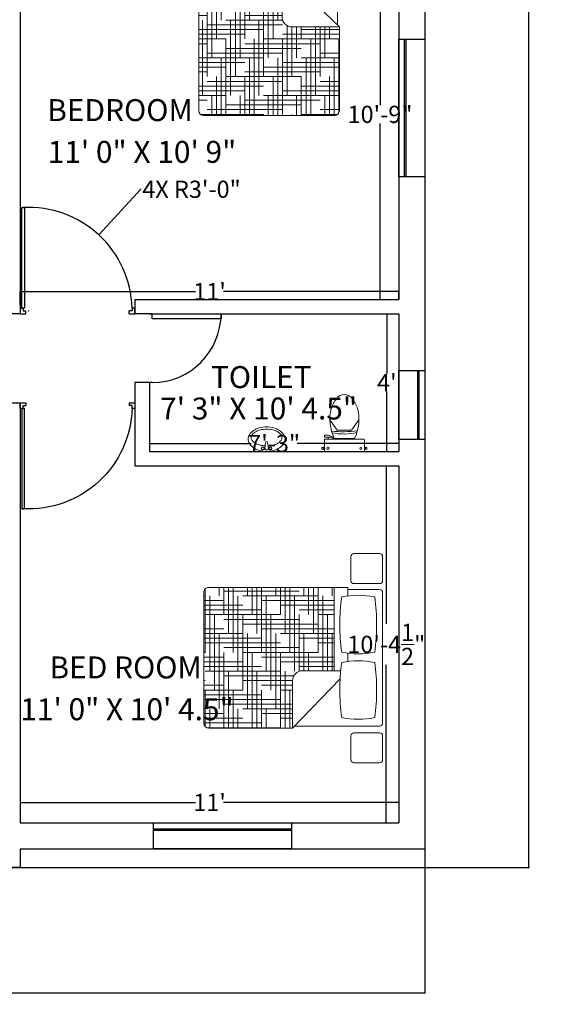
# Model space of a CAD drawing. Units: inches. Extents: x -113 to 5399, y -1393 to 3302.
# Tile 26 of 40: x 3982 to 4170, y -154 to 189. Entities that reach past the tile are written whole.
import ezdxf

# ---------------------------------------------------------------- set-up
doc = ezdxf.new("R2010")
doc.units = ezdxf.units.IN
doc.header["$MEASUREMENT"] = 0
for name, color, linetype, lineweight in [('A-ANNO-DIMS', 254, 'Continuous', 18), ('A-AREA-IDEN', 4, 'Continuous', 18), ('A-FLOR-FIXT', 8, 'Continuous', 18), ('doors', 2, 'Continuous', 25), ('furniture', 131, 'Continuous', 18), ('walls', 1, 'Continuous', 25), ('windows', 3, 'Continuous', 25)]:
    doc.layers.add(name, color=color, linetype=linetype, lineweight=lineweight)
doc.layers.add('A-GLAZ-PATT', color=85, linetype='Continuous', lineweight=13, true_color=0x58ba48)
doc.styles.get("Standard").update_dxf_attribs({"font": 'arial.ttf'})
doc.dimstyles.get("Standard").update_dxf_attribs({"dimtxt": 6, "dimasz": 0.18, "dimexe": 0.18, "dimexo": 0.0625, "dimgap": 0.09, "dimtad": 0, "dimtih": 1, "dimtoh": 1, "dimdec": 1, "dimzin": 0, "dimdsep": 46, "dimlunit": 4, "dimtxsty": 'Standard', "dimblk": 'ARCHTICK', "dimcen": 0.09, "dimadec": 0, "dimazin": 0, "dimtfac": 1, "dimtdec": 1, "dimtofl": 0, "dimtmove": 0, "dimatfit": 3, "dimfxl": 1, "dimtolj": 1, "dimtzin": 0, "dimarcsym": 0})

# ---------------------------------------------------------------- blocks, each defined once
blk = doc.blocks.new('*U2')
for p, q in [((0, 0), (0, -6)), ((24, 0), (24, -6))]:
    blk.add_line(p, q)
blk.add_lwpolyline([(0, 0), (0, 24), (1.75, 24), (1.75, 0)], close=True)
blk.add_arc((0, 0), 24, 0, 90)
blk = doc.blocks.new('*X4')
at = {"color": 0}
for p, q in [((4.3594, 18.5625), (4.3594, 18.6457)), ((4.5, 18), (4.5, 18.6457)), ((4.5469, 18.1875), (4.5469, 18.6457)), ((4.5938, 18.375), (4.5938, 18.6457)), ((4.6406, 18.5625), (4.6406, 18.6457)), ((4.7812, 18), (4.7812, 18.6457)), ((4.8281, 18.1875), (4.8281, 18.6457)), ((4.875, 18.375), (4.875, 18.6457)), ((4.9219, 18.5625), (4.9219, 18.6457)), ((5.0625, 18), (5.0625, 18.6457)), ((5.1094, 18.1875), (5.1094, 18.6457)), ((5.1562, 18.375), (5.1562, 18.6457)), ((5.2031, 18.5625), (5.2031, 18.6457)), ((5.3438, 18), (5.3438, 18.6457)), ((5.3906, 18.1875), (5.3906, 18.6457)), ((5.4375, 18.375), (5.4375, 18.6457)), ((5.4844, 18.5625), (5.4844, 18.6457)), ((5.625, 18), (5.625, 18.6287)), ((4.4531, 17.8169), (4.4531, 18.5625)), ((4.5, 18.5625), (5.25, 18.5625)), ((4.6875, 18.6094), (5.4375, 18.6094)), ((4.7344, 17.8125), (4.7344, 18.5625)), ((5.0156, 17.8125), (5.0156, 18.5625)), ((5.2969, 17.8125), (5.2969, 18.5625)), ((5.5781, 17.8125), (5.5781, 18.5625)), ((5.625, 18.5625), (5.6375, 18.5625)), ((4.3395, 18.5156), (5.0625, 18.5156)), ((4.3395, 18.4688), (4.875, 18.4688)), ((5.25, 18.4688), (5.6375, 18.4688)), ((5.4375, 18.5156), (5.6375, 18.5156)), ((4.3395, 18.4219), (4.6875, 18.4219)), ((4.3395, 18.375), (4.5, 18.375)), ((4.4062, 17.8169), (4.4062, 18.375)), ((4.6875, 17.8114), (4.6875, 18.375)), ((4.6875, 18.3281), (5.4375, 18.3281)), ((4.875, 18.375), (5.625, 18.375)), ((4.9688, 17.625), (4.9688, 18.375)), ((5.0625, 18.4219), (5.6375, 18.4219)), ((5.25, 17.625), (5.25, 18.375)), ((5.5312, 17.625), (5.5312, 18.375)), ((4.3395, 18.2344), (5.0625, 18.2344)), ((4.5, 18.2812), (5.25, 18.2812)), ((5.4375, 18.2344), (5.6375, 18.2344)), ((5.625, 18.2812), (5.6375, 18.2812)), ((4.3395, 18.1875), (4.875, 18.1875)), ((4.3395, 18.1406), (4.6875, 18.1406)), ((4.3594, 17.8169), (4.3594, 18.1875)), ((4.6406, 17.8169), (4.6406, 18.1875)), ((4.9219, 17.4375), (4.9219, 18.1875)), ((5.0625, 18.1406), (5.6375, 18.1406)), ((5.2031, 17.4375), (5.2031, 18.1875)), ((5.25, 18.1875), (5.6375, 18.1875)), ((5.4844, 17.4375), (5.4844, 18.1875)), ((4.3395, 18.0938), (4.5, 18.0938)), ((4.6875, 18.0469), (5.4375, 18.0469)), ((4.875, 18.0938), (5.625, 18.0938)), ((4.3395, 17.9531), (5.0625, 17.9531)), ((4.5, 18), (5.25, 18)), ((4.5938, 17.8169), (4.5938, 18)), ((4.875, 17.25), (4.875, 18)), ((5.1562, 17.25), (5.1562, 18)), ((5.4375, 17.25), (5.4375, 18)), ((5.4375, 17.9531), (5.6375, 17.9531)), ((5.625, 18), (5.6375, 18)), ((4.3395, 17.9062), (4.875, 17.9062)), ((4.3395, 17.8594), (4.6875, 17.8594)), ((5.0625, 17.8594), (5.6375, 17.8594)), ((5.25, 17.9062), (5.6375, 17.9062)), ((4.7421, 17.7656), (5.4375, 17.7656)), ((4.8281, 17.2457), (4.8281, 17.8125)), ((4.875, 17.8125), (5.625, 17.8125)), ((5.1094, 17.2457), (5.1094, 17.8125)), ((5.3906, 17.2457), (5.3906, 17.8125)), ((4.7548, 17.7188), (5.25, 17.7188)), ((4.7548, 17.6719), (5.0625, 17.6719)), ((5.4375, 17.6719), (5.6375, 17.6719)), ((5.625, 17.7188), (5.6375, 17.7188)), ((4.7548, 17.625), (4.875, 17.625)), ((4.7812, 17.2457), (4.7812, 17.625)), ((5.0625, 17.2457), (5.0625, 17.625)), ((5.0625, 17.5781), (5.6375, 17.5781)), ((5.25, 17.625), (5.6375, 17.625)), ((5.3438, 17.2457), (5.3438, 17.625)), ((5.625, 17.2627), (5.625, 17.625)), ((4.7548, 17.4844), (5.4375, 17.4844)), ((4.875, 17.5312), (5.625, 17.5312)), ((4.7548, 17.4375), (5.25, 17.4375)), ((4.7548, 17.3906), (5.0625, 17.3906)), ((5.0156, 17.2457), (5.0156, 17.4375)), ((5.2969, 17.2457), (5.2969, 17.4375)), ((5.4375, 17.3906), (5.6375, 17.3906)), ((5.5781, 17.2457), (5.5781, 17.4375)), ((5.625, 17.4375), (5.6375, 17.4375)), ((4.7548, 17.3438), (4.875, 17.3438)), ((4.875, 17.25), (5.6077, 17.25)), ((4.9688, 17.2457), (4.9688, 17.25)), ((5.0625, 17.2969), (5.6375, 17.2969)), ((5.25, 17.3438), (5.6375, 17.3438)), ((5.25, 17.2457), (5.25, 17.25)), ((5.5312, 17.2457), (5.5312, 17.25))]:
    blk.add_line(p, q, dxfattribs=at)
blk = doc.blocks.new('MAT-P01')
for p, q in [((-0.0213, 0.8164), (-0.0213, 0.5605)), ((0.0087, 0.8464), (0.2471, 0.8464)), ((0.2771, 0.8164), (0.2771, 0.5605)), ((0.3437, 0.8164), (0.3437, -0.0316)), ((0.3737, 0.8464), (1.6737, 0.8464)), ((1.7037, 0.8164), (1.7037, 0.5005)), ((1.7622, 0.8164), (1.7622, 0.5605)), ((1.7922, 0.8464), (2.0306, 0.8464)), ((2.0606, 0.8164), (2.0606, 0.5605)), ((0.0087, 0.5305), (0.2471, 0.5305)), ((0.9879, 0.5005), (1.0693, 0.5005)), ((1.6393, 0.5005), (1.7237, 0.5005)), ((1.7237, 0.5005), (1.7237, -0.8836)), ((1.7922, 0.5305), (2.0306, 0.5305)), ((0.8146, 0.423), (0.3237, -0.0509)), ((0.8949, 0.4293), (0.8949, 0.0491)), ((0.8949, 0.3643), (1.7237, 0.3643)), ((0.8949, 0.3643), (0.8949, 0.0491)), ((0.8949, 0.3643), (1.7237, 0.3643)), ((1.7237, 0.3643), (1.7237, -0.8836)), ((0.3237, -0.0509), (0.7949, -0.0509)), ((0.3237, -0.0509), (0.3237, -0.8836)), ((0.3737, -0.9336), (1.6737, -0.9336))]:
    blk.add_line(p, q)
for centre, radius, start, end in [((0.0087, 0.8164), 0.03, 90, 180), ((0.2471, 0.8164), 0.03, 0, 90), ((0.3737, 0.8164), 0.03, 90, 180), ((0.7029, -1.1436), 1.9306, 81.81622, 98.18378), ((1.3543, -1.1436), 1.9306, 81.81622, 98.18378), ((1.6737, 0.8164), 0.03, 0, 90), ((1.7922, 0.8164), 0.03, 90, 180), ((2.0306, 0.8164), 0.03, 0, 90), ((1.2251, 0.6034), 0.8138, 168.37298, 191.62702), ((0.1806, 0.6034), 0.8138, 348.37298, 11.62702), ((1.8766, 0.6034), 0.8138, 168.37298, 191.62702), ((0.8321, 0.6034), 0.8138, 348.37298, 11.62702), ((0.0087, 0.5605), 0.03, 180, 270), ((0.2471, 0.5605), 0.03, 270, 0), ((1.7922, 0.5605), 0.03, 180, 270), ((2.0306, 0.5605), 0.03, 270, 0), ((0.7029, 2.3504), 1.9306, 261.81622, 278.18378), ((1.3543, 2.3504), 1.9306, 261.81622, 278.18378), ((0.7949, 0.0491), 0.1, 270, 0), ((0.3737, -0.8836), 0.05, 180, 270), ((1.6737, -0.8836), 0.05, 270, 0)]:
    blk.add_arc(centre, radius, start, end)
at = {"rotation": 270}
blk.add_blockref('*X4', (-16.9221, 4.7038), dxfattribs=at)
blk = doc.blocks.new('toilet-3')
at = {"color": 0, "linetype": 'ByBlock'}
for p, q in [((-0.281, -0.05), (-0.281, -0.069)), ((-0.281, -0.05), (-0.261, -0.05)), ((-0.281, -0.069), (-0.261, -0.069)), ((-0.261, -0.047), (-0.261, -0.072)), ((-0.261, -0.047), (-0.251, -0.047)), ((-0.261, -0.072), (-0.251, -0.072)), ((-0.251, -0.047), (-0.251, -0.072)), ((-0.25, -0.03), (-0.25, -0.165)), ((0.24, -0.02), (-0.24, -0.02)), ((0.25, -0.03), (0.25, -0.165)), ((0.261, -0.047), (0.251, -0.047)), ((0.251, -0.047), (0.251, -0.072)), ((0.261, -0.072), (0.251, -0.072)), ((0.261, -0.047), (0.261, -0.072)), ((0.281, -0.05), (0.261, -0.05)), ((0.281, -0.069), (0.261, -0.069)), ((0.281, -0.05), (0.281, -0.069)), ((-0.144, -0.2), (-0.25, -0.2)), ((-0.25, -0.2), (-0.25, -0.222)), ((-0.198, -0.222), (-0.25, -0.222)), ((0.24, -0.175), (-0.24, -0.175)), ((-0.202, -0.2), (-0.202, -0.175)), ((-0.198, -0.222), (-0.16, -0.207)), ((-0.16, -0.207), (-0.16, -0.2)), ((-0.144, -0.2), (-0.144, -0.175)), ((0.125, -0.182), (-0.125, -0.182)), ((-0.089, -0.287), (-0.18, -0.415)), ((0.089, -0.287), (-0.089, -0.287)), ((0.089, -0.287), (0.18, -0.415))]:
    blk.add_line(p, q, dxfattribs=at)
for centre in [(-0.205, -0.059), (0.205, -0.059)]:
    blk.add_circle(centre, 0.0125, dxfattribs=at)
for centre, radius, start, end in [((-0.24, -0.03), 0.01, 90, 180), ((0.24, -0.03), 0.01, 0, 90), ((-0.24, -0.165), 0.01, 180, 270), ((0.376, -0.424), 0.557, 154.2321, 193.6755), ((-0.005, -0.896), 0.659, 75.9276, 103.0204), ((-0.376, -0.424), 0.557, 346.3245, 25.7679), ((0.24, -0.165), 0.01, 270, 0), ((-0.013, -1.787), 1.521, 83.4552, 95.5271), ((0.262, -0.406), 0.452, 199.2942, 217.2549), ((-0.265, -0.4), 0.457, 322.2382, 340.1051), ((-0.001, -0.609), 0.12, 216.3794, 323.6206)]:
    blk.add_arc(centre, radius, start, end, dxfattribs=at)
blk = doc.blocks.new('wash-6')
at = {"color": 0, "linetype": 'ByBlock'}
for p, q in [((-0.036, -0.063), (-0.021, -0.18)), ((0.036, -0.063), (0.021, -0.18))]:
    blk.add_line(p, q, dxfattribs=at)
for centre, radius in [((-0.075, -0.062), 0.0325), ((-0.075, -0.062), 0.0263), ((0.075, -0.062), 0.0325), ((0.075, -0.062), 0.0263)]:
    blk.add_circle(centre, radius, dxfattribs=at)
for centre, radius, start, end in [((0, -0.56), 0.56, 90, 105.4371), ((-0.204, -0.25), 0.17, 148.1465, 180), ((-0.107, -0.311), 0.285, 123.6901, 148.1465), ((-0.114, -0.361), 0.225, 118.369, 142.5096), ((-0.042, -0.407), 0.401, 105.4371, 123.6901), ((-0.045, -0.488), 0.37, 102.6081, 118.369), ((0, -0.69), 0.576, 92.9466, 102.6081), ((0, -0.063), 0.0361, 0, 180), ((0, -0.18), 0.0215, 180, 0), ((0, -0.56), 0.56, 74.5629, 90), ((0, -0.69), 0.576, 77.3919, 87.0534), ((0.045, -0.488), 0.37, 61.631, 77.3919), ((0.042, -0.407), 0.401, 56.3099, 74.5629), ((0.114, -0.361), 0.225, 37.4904, 61.631), ((0.107, -0.311), 0.285, 31.8535, 56.3099), ((0.204, -0.25), 0.17, 0, 31.8535), ((-0.204, -0.25), 0.17, 180, 211.8535), ((-0.107, -0.189), 0.285, 211.8535, 236.3099), ((-0.217, -0.282), 0.0954, 142.5096, 180), ((-0.217, -0.282), 0.0954, 180, 217.4904), ((-0.114, -0.203), 0.225, 217.4904, 241.631), ((0.114, -0.203), 0.225, 298.369, 322.5096), ((0.107, -0.189), 0.285, 303.6901, 328.1465), ((0.217, -0.282), 0.0954, 0, 37.4904), ((0.217, -0.282), 0.0954, 322.5096, 0), ((0.204, -0.25), 0.17, 328.1465, 0), ((-0.042, -0.092), 0.401, 236.3099, 254.5629), ((-0.045, -0.076), 0.37, 241.631, 257.3919), ((0, 0.06), 0.56, 254.5629, 270), ((0, 0.125), 0.576, 257.3919, 270), ((0, 0.125), 0.576, 270, 282.6081), ((0, 0.06), 0.56, 270, 285.4371), ((0.045, -0.076), 0.37, 282.6081, 298.369), ((0.042, -0.092), 0.401, 285.4371, 303.6901)]:
    blk.add_arc(centre, radius, start, end, dxfattribs=at)
blk = doc.blocks.new('_ArchTick')
at = {"color": 0, "linetype": 'ByBlock', "const_width": 0.15}
blk.add_lwpolyline([(-0.5, -0.5), (0.5, 0.5)], dxfattribs=at)
blk = doc.blocks.new('*D99')
at = {"layer": 'A-ANNO-DIMS', "color": 0, "lineweight": -2, "transparency": 16777216}
for p, q in [((3689.73, -100.29), (3689.73, -150.66)), ((4122.73, -100.29), (4122.73, -150.66)), ((3689.73, -150.48), (3895.84, -150.48)), ((4122.73, -150.48), (3916.62, -150.48))]:
    blk.add_line(p, q, dxfattribs=at)
at = {"layer": 'Defpoints', "color": 0, "transparency": 16777216}
for p in [(3689.73, -100.22), (4122.73, -100.22), (4122.73, -150.48)]:
    blk.add_point(p, dxfattribs=at)
at = {"layer": 'A-ANNO-DIMS', "color": 0, "lineweight": -2, "transparency": 16777216, "xscale": 0.18, "yscale": 0.18, "zscale": 0.18, "rotation": 180}
blk.add_blockref('_ArchTick', (3689.73, -150.48), dxfattribs=at)
at = {"layer": 'A-ANNO-DIMS', "color": 0, "lineweight": -2, "transparency": 16777216, "xscale": 0.18, "yscale": 0.18, "zscale": 0.18}
blk.add_blockref('_ArchTick', (4122.73, -150.48), dxfattribs=at)
at = {"layer": 'A-ANNO-DIMS', "color": 0, "transparency": 16777216, "insert": (3906.23, -150.48), "char_height": 6, "attachment_point": 5}
blk.add_mtext('\\A1;36\'-1"', dxfattribs=at)
blk = doc.blocks.new('*D103')
at = {"layer": 'A-ANNO-DIMS', "color": 0, "lineweight": -2, "transparency": 16777216}
for p, q in [((4107.42, 220.28), (4106.96, 220.28)), ((4107.14, 220.28), (4107.14, 158.93)), ((4107.14, 91.28), (4107.14, 152.62)), ((4107.42, 91.28), (4106.96, 91.28))]:
    blk.add_line(p, q, dxfattribs=at)
at = {"layer": 'Defpoints', "color": 0, "transparency": 16777216}
for p in [(4107.48, 220.28), (4107.14, 91.28), (4107.48, 91.28)]:
    blk.add_point(p, dxfattribs=at)
at = {"layer": 'A-ANNO-DIMS', "color": 0, "lineweight": -2, "transparency": 16777216, "xscale": 0.18, "yscale": 0.18, "zscale": 0.18}
for p, rotation in [((4107.14, 220.28), 90), ((4107.14, 91.28), 270)]:
    blk.add_blockref('_ArchTick', p, dxfattribs=dict(at, rotation=rotation))
at = {"layer": 'A-ANNO-DIMS', "color": 0, "transparency": 16777216, "insert": (4107.14, 155.78), "char_height": 6, "attachment_point": 5}
blk.add_mtext('\\A1;10\'-9"', dxfattribs=at)
blk = doc.blocks.new('*D104')
at = {"layer": 'A-ANNO-DIMS', "color": 0, "lineweight": -2, "transparency": 16777216}
for p, q in [((3981.73, 89.33), (3981.73, 94.18)), ((3981.73, 94), (4042.83, 94)), ((4113.73, 94), (4052.63, 94)), ((4113.73, 91.34), (4113.73, 94.18))]:
    blk.add_line(p, q, dxfattribs=at)
at = {"layer": 'Defpoints', "color": 0, "transparency": 16777216}
for p in [(4113.73, 94), (3981.73, 89.26), (4113.73, 91.28)]:
    blk.add_point(p, dxfattribs=at)
at = {"layer": 'A-ANNO-DIMS', "color": 0, "lineweight": -2, "transparency": 16777216, "xscale": 0.18, "yscale": 0.18, "zscale": 0.18, "rotation": 180}
blk.add_blockref('_ArchTick', (3981.73, 94), dxfattribs=at)
at = {"layer": 'A-ANNO-DIMS', "color": 0, "lineweight": -2, "transparency": 16777216, "xscale": 0.18, "yscale": 0.18, "zscale": 0.18}
blk.add_blockref('_ArchTick', (4113.73, 94), dxfattribs=at)
at = {"layer": 'A-ANNO-DIMS', "color": 0, "transparency": 16777216, "insert": (4047.73, 94), "char_height": 6, "attachment_point": 5}
blk.add_mtext("\\A1;11'", dxfattribs=at)
blk = doc.blocks.new('*D105')
at = {"layer": 'A-ANNO-DIMS', "color": 0, "lineweight": -2, "transparency": 16777216}
for p, q in [((4109.32, 86.28), (4109.69, 86.28)), ((4109.51, 86.28), (4109.51, 65.37)), ((4109.51, 38.28), (4109.51, 59.19)), ((4109.32, 38.28), (4109.69, 38.28))]:
    blk.add_line(p, q, dxfattribs=at)
at = {"layer": 'Defpoints', "color": 0, "transparency": 16777216}
for p in [(4109.25, 86.28), (4109.25, 38.28), (4109.51, 38.28)]:
    blk.add_point(p, dxfattribs=at)
at = {"layer": 'A-ANNO-DIMS', "color": 0, "lineweight": -2, "transparency": 16777216, "xscale": 0.18, "yscale": 0.18, "zscale": 0.18}
for p, rotation in [((4109.51, 86.28), 90), ((4109.51, 38.28), 270)]:
    blk.add_blockref('_ArchTick', p, dxfattribs=dict(at, rotation=rotation))
at = {"layer": 'A-ANNO-DIMS', "color": 0, "transparency": 16777216, "insert": (4109.51, 62.28), "char_height": 6, "attachment_point": 5}
blk.add_mtext("\\A1;4'", dxfattribs=at)
blk = doc.blocks.new('*D106')
at = {"layer": 'A-ANNO-DIMS', "color": 0, "lineweight": -2, "transparency": 16777216}
for p, q in [((4026.73, 41.09), (4026.73, 41.21)), ((4113.73, 41.09), (4113.73, 41.21)), ((4026.73, 41.03), (4062.19, 41.03)), ((4113.73, 41.03), (4078.27, 41.03))]:
    blk.add_line(p, q, dxfattribs=at)
at = {"layer": 'Defpoints', "color": 0, "transparency": 16777216}
for p in [(4026.73, 41.03), (4113.73, 41.03), (4113.73, 41.03)]:
    blk.add_point(p, dxfattribs=at)
at = {"layer": 'A-ANNO-DIMS', "color": 0, "lineweight": -2, "transparency": 16777216, "xscale": 0.18, "yscale": 0.18, "zscale": 0.18, "rotation": 180}
blk.add_blockref('_ArchTick', (4026.73, 41.03), dxfattribs=at)
at = {"layer": 'A-ANNO-DIMS', "color": 0, "lineweight": -2, "transparency": 16777216, "xscale": 0.18, "yscale": 0.18, "zscale": 0.18}
blk.add_blockref('_ArchTick', (4113.73, 41.03), dxfattribs=at)
at = {"layer": 'A-ANNO-DIMS', "color": 0, "transparency": 16777216, "insert": (4070.23, 41.03), "char_height": 6, "attachment_point": 5}
blk.add_mtext('\\A1;7\'-3"', dxfattribs=at)
blk = doc.blocks.new('*D119')
at = {"layer": 'A-ANNO-DIMS', "color": 0, "lineweight": -2, "transparency": 16777216}
for p, q in [((4108.21, 33.28), (4109.51, 33.28)), ((4109.33, 33.28), (4109.33, -21.81)), ((4109.33, -91.22), (4109.33, -36.14)), ((4108.21, -91.22), (4109.51, -91.22))]:
    blk.add_line(p, q, dxfattribs=at)
at = {"layer": 'Defpoints', "color": 0, "transparency": 16777216}
for p in [(4108.15, 33.28), (4108.15, -91.22), (4109.33, -91.22)]:
    blk.add_point(p, dxfattribs=at)
at = {"layer": 'A-ANNO-DIMS', "color": 0, "lineweight": -2, "transparency": 16777216, "xscale": 0.18, "yscale": 0.18, "zscale": 0.18}
for p, rotation in [((4109.33, 33.28), 90), ((4109.33, -91.22), 270)]:
    blk.add_blockref('_ArchTick', p, dxfattribs=dict(at, rotation=rotation))
at = {"layer": 'A-ANNO-DIMS', "color": 0, "transparency": 16777216, "insert": (4109.33, -28.97), "char_height": 6, "attachment_point": 5}
blk.add_mtext('\\A1;10\'-4{\\H1x;\\S1/2;}"', dxfattribs=at)
blk = doc.blocks.new('*D120')
at = {"layer": 'A-ANNO-DIMS', "color": 0, "lineweight": -2, "transparency": 16777216}
for p, q in [((3981.73, -83.95), (3981.73, -84.23)), ((3981.73, -84.05), (4042.83, -84.05)), ((4113.73, -84.05), (4052.63, -84.05)), ((4113.73, -83.95), (4113.73, -84.23))]:
    blk.add_line(p, q, dxfattribs=at)
at = {"layer": 'Defpoints', "color": 0, "transparency": 16777216}
for p in [(3981.73, -83.88), (4113.73, -83.88), (4113.73, -84.05)]:
    blk.add_point(p, dxfattribs=at)
at = {"layer": 'A-ANNO-DIMS', "color": 0, "lineweight": -2, "transparency": 16777216, "xscale": 0.18, "yscale": 0.18, "zscale": 0.18, "rotation": 180}
blk.add_blockref('_ArchTick', (3981.73, -84.05), dxfattribs=at)
at = {"layer": 'A-ANNO-DIMS', "color": 0, "lineweight": -2, "transparency": 16777216, "xscale": 0.18, "yscale": 0.18, "zscale": 0.18}
blk.add_blockref('_ArchTick', (4113.73, -84.05), dxfattribs=at)
at = {"layer": 'A-ANNO-DIMS', "color": 0, "transparency": 16777216, "insert": (4047.73, -84.05), "char_height": 6, "attachment_point": 5}
blk.add_mtext("\\A1;11'", dxfattribs=at)
blk = doc.blocks.new('WIN-PLAN-48IN')
h = blk.add_hatch(color=256)
h.dxf.hatch_style = 1
h.paths.add_polyline_path([(48, 2.5), (0, 2.5), (0, 2), (48, 2)])
for p, q in [((0, 9), (48, 9)), ((0, 0), (0, 9)), ((48, 9), (48, 0)), ((48, 2.5), (0, 2.5)), ((48, 2), (0, 2)), ((48, 0), (0, 0))]:
    blk.add_line(p, q)
blk = doc.blocks.new('DOOR-SINGLE-36IN-PLAN')
for p, q in [((0.5, 2), (0.5, 36.98)), ((0.5, 36.98), (1.5, 36.98)), ((1.5, 36.98), (1.5, 2)), ((0, 2), (0, 0)), ((0, 2), (1.04, 2)), ((1.5, 2), (0.5, 2)), ((1.04, 2), (1.04, 0.98)), ((1.04, 0.98), (2, 0.98)), ((2, 0), (2, 0.98)), ((38.96, 0.98), (38, 0.98)), ((38, 0), (38, 0.98)), ((40, 2), (38.96, 2)), ((38.96, 2), (38.96, 0.98)), ((40, 0), (40, 2)), ((0, 0), (2, 0)), ((0, 0), (2, 0)), ((38, 0), (40, 0))]:
    blk.add_line(p, q)
blk.add_arc((2.94, 0.99), 36.04, 1.6003, 93.0893)
blk = doc.blocks.new('*D210')
at = {"layer": 'A-ANNO-DIMS', "color": 0, "lineweight": -2, "transparency": 16777216}
for p, q in [((3839.79, 561.28), (4159.21, 561.28)), ((4159.03, 561.28), (4159.03, 230.43)), ((4159.03, -106.72), (4159.03, 224.12)), ((3839.79, -106.72), (4159.21, -106.72))]:
    blk.add_line(p, q, dxfattribs=at)
at = {"layer": 'Defpoints', "color": 0, "transparency": 16777216}
for p in [(3839.73, 561.28), (4159.03, 561.28), (3839.73, -106.72)]:
    blk.add_point(p, dxfattribs=at)
at = {"layer": 'A-ANNO-DIMS', "color": 0, "lineweight": -2, "transparency": 16777216, "xscale": 0.18, "yscale": 0.18, "zscale": 0.18}
for p, rotation in [((4159.03, 561.28), 90), ((4159.03, -106.72), 270)]:
    blk.add_blockref('_ArchTick', p, dxfattribs=dict(at, rotation=rotation))
at = {"layer": 'A-ANNO-DIMS', "color": 0, "transparency": 16777216, "insert": (4159.03, 227.28), "char_height": 6, "attachment_point": 5}
blk.add_mtext('\\A1;55\'-8"', dxfattribs=at)
blk = doc.blocks.new('*D240')
at = {"layer": 'A-ANNO-DIMS', "color": 0, "lineweight": -2, "transparency": 16777216}
for p, q in [((4023.74, 129.67), (4009.09, 113.77)), ((4023.92, 129.67), (4023.74, 129.67)), ((3984.58, 87.27), (3984.76, 87.27)), ((3984.67, 87.18), (3984.67, 87.36))]:
    blk.add_line(p, q, dxfattribs=at)
at = {"layer": 'Defpoints', "color": 0, "transparency": 16777216}
for p in [(4009.09, 113.77), (3984.67, 87.27)]:
    blk.add_point(p, dxfattribs=at)
at = {"layer": 'A-ANNO-DIMS', "color": 0, "lineweight": -2, "transparency": 16777216, "xscale": 0.18, "yscale": 0.18, "zscale": 0.18, "rotation": 227.3452027332481}
blk.add_blockref('_ArchTick', (4009.09, 113.77), dxfattribs=at)
at = {"layer": 'A-ANNO-DIMS', "color": 0, "transparency": 16777216, "insert": (4041.42, 129.67), "char_height": 6, "attachment_point": 5}
blk.add_mtext('\\A1;4X R3\'-0"', dxfattribs=at)

msp = doc.modelspace()

# ---------------------------------------------------------------- hatches: boundary and pattern name
at = {"layer": 'A-GLAZ-PATT'}
h = msp.add_hatch(color=256, dxfattribs=at)
h.dxf.hatch_style = 1
h.paths.add_polyline_path([(4120.23, 66.46), (4120.23, 42.46), (4120.73, 42.46), (4120.73, 66.46)])

# ---------------------------------------------------------------- linework, layer by layer
at = {"layer": 'walls'}
for p, q in [((4122.73, 549.78), (4122.73, -100.22)), ((3981.73, 220.28), (3981.73, 88.28)), ((4113.73, 220.28), (4113.73, 95.78)), ((4113.73, 95.78), (4113.73, 91.28)), ((4021.73, 91.28), (4021.73, 86.28)), ((4021.73, 91.28), (4113.73, 91.28)), ((3981.73, 86.28), (3976.73, 86.28)), ((4026.73, 86.28), (4021.73, 86.28)), ((4026.73, 86.28), (4113.73, 86.28)), ((4113.73, 86.28), (4113.73, 38.28)), ((4021.73, 62.28), (4021.73, 33.28)), ((4026.73, 62.28), (4021.73, 62.28)), ((4026.73, 62.28), (4026.73, 38.28)), ((3976.73, 55.28), (3981.73, 55.28)), ((3981.73, 55.28), (3981.73, -91.22)), ((4026.73, 38.28), (4113.73, 38.28)), ((4021.73, 33.28), (4113.73, 33.28)), ((4113.73, 33.28), (4113.73, -91.22)), ((3981.73, -91.22), (4113.73, -91.22)), ((3981.73, -100.22), (4122.73, -100.22)), ((3981.73, -100.22), (3981.73, -106.72)), ((3981.73, -106.72), (3976.73, -106.72))]:
    msp.add_line(p, q, dxfattribs=at)
at = {"layer": 'windows'}
for p, q in [((4113.73, 42.46), (4113.73, 66.46)), ((4113.73, 66.46), (4122.73, 66.46)), ((4120.23, 66.46), (4120.23, 42.46)), ((4120.73, 66.46), (4120.73, 42.46)), ((4122.73, 66.46), (4122.73, 42.46)), ((4122.73, 42.46), (4113.73, 42.46))]:
    msp.add_line(p, q, dxfattribs=at)

# ---------------------------------------------------------------- block references
at = {"layer": 'A-FLOR-FIXT', "rotation": 180}
for name, p, xscale, yscale, zscale in [('toilet-3', (4094.73, 37.72), -27.95492935005888, 27.95492935005888, 27.95492935005888), ('wash-6', (4067.61, 38.28), -17.16666334294967, 17.16666334294967, 17.16666334294967)]:
    msp.add_blockref(name, p, dxfattribs=dict(at, xscale=xscale, yscale=yscale, zscale=zscale))
at = {"layer": 'doors'}
msp.add_blockref('DOOR-SINGLE-36IN-PLAN', (3981.73, 86.28), dxfattribs=at)
at = {"layer": 'doors', "rotation": 270}
msp.add_blockref('*U2', (4027.73, 86.28), dxfattribs=at)
at = {"layer": 'doors', "extrusion": (0, 0, -1), "zscale": -1, "rotation": 180}
msp.add_blockref('DOOR-SINGLE-36IN-PLAN', (-3981.73, 55.28), dxfattribs=at)
at = {"layer": 'furniture', "xscale": -35.02364872074636, "yscale": 35.02364872074636, "zscale": 35.02364872074636}
msp.add_blockref('MAT-P01', (4104.32, 188.05), dxfattribs=at)
at = {"layer": 'furniture', "xscale": -35.02364872074636, "yscale": 35.02364872074636, "zscale": 35.02364872074636, "rotation": 270}
msp.add_blockref('MAT-P01', (4078.41, -69.49), dxfattribs=at)
at = {"layer": 'windows'}
for p, rotation in [((4113.73, 182.03), 270.0000000000004), ((4076.23, -91.22), 180)]:
    msp.add_blockref('WIN-PLAN-48IN', p, dxfattribs=dict(at, rotation=rotation))

# ---------------------------------------------------------------- texts
at = {"layer": 'A-AREA-IDEN'}
for s, height, p in [('BEDROOM', 7.647, (3991.12, 153.43)), ('11\' 0" X 10\' 9"', 7.6473, (3991.29, 138.88)), ('TOILET', 7.647, (4048.2, 60.38)), ('7\' 3" X 10\' 4.5"', 7.6473, (4030.49, 49.42)), ('BED ROOM', 7.647, (3991.92, -40.82)), ('11\' 0" X 10\' 4.5"', 7.6473, (3981.73, -55.39))]:
    msp.add_text(s, height=height, dxfattribs=at).set_placement(p)

# ---------------------------------------------------------------- dimensions: what is measured, and where the dimension line sits
at = {"layer": 'A-ANNO-DIMS'}
for base, p1, p2, override, picture, middle in [((4159.03, 561.28), (3839.73, -106.72), (3839.73, 561.28), {"dimdec": 1, "dimlfac": 1, "dimrnd": 0, "dimzin": 1, "dimdsep": 46, "dimlunit": 4, "dimfrac": 2}, '*D210', (4159.03, 227.28)), ((4107.14, 91.28), (4107.48, 220.28), (4107.48, 91.28), {"dimclrd": 0, "dimclre": 0, "dimclrt": 0}, '*D103', (4107.14, 155.78)), ((4109.51, 38.28), (4109.25, 86.28), (4109.25, 38.28), {"dimclrd": 0, "dimclre": 0, "dimclrt": 0}, '*D105', (4109.51, 62.28)), ((4109.33, -91.22), (4108.15, 33.28), (4108.15, -91.22), {"dimclrd": 0, "dimclre": 0, "dimclrt": 0}, '*D119', (4109.33, -28.97))]:
    dim = msp.add_linear_dim(base=base, p1=p1, p2=p2, angle=90, dimstyle='Standard', override=override, dxfattribs=at)
    dim.commit()
    dim.dimension.update_dxf_attribs({"geometry": picture, "text_midpoint": middle})
dim = msp.add_radius_dim(center=(3984.67, 87.27), mpoint=(4009.09, 113.77), text='4X <>', dimstyle='Standard', override={"dimdec": 1, "dimlfac": 1, "dimrnd": 0, "dimzin": 1, "dimdsep": 46, "dimlunit": 4, "dimfrac": 2}, dxfattribs=at)
dim.commit()
dim.dimension.update_dxf_attribs({"geometry": '*D240', "text_midpoint": (4041.42, 129.67), "dimtype": 164})
for base, p1, p2, picture, middle in [((4113.73, 94), (3981.73, 89.26), (4113.73, 91.28), '*D104', (4047.73, 94)), ((4113.73, 41.03), (4026.73, 41.03), (4113.73, 41.03), '*D106', (4070.23, 41.03)), ((4113.73, -84.05), (3981.73, -83.88), (4113.73, -83.88), '*D120', (4047.73, -84.05)), ((4122.73, -150.48), (3689.73, -100.22), (4122.73, -100.22), '*D99', (3906.23, -150.48))]:
    dim = msp.add_linear_dim(base=base, p1=p1, p2=p2, dimstyle='Standard', override={"dimclrd": 0, "dimclre": 0, "dimclrt": 0}, dxfattribs=at)
    dim.commit()
    dim.dimension.update_dxf_attribs({"geometry": picture, "text_midpoint": middle})

doc.saveas('drawing.dxf')
